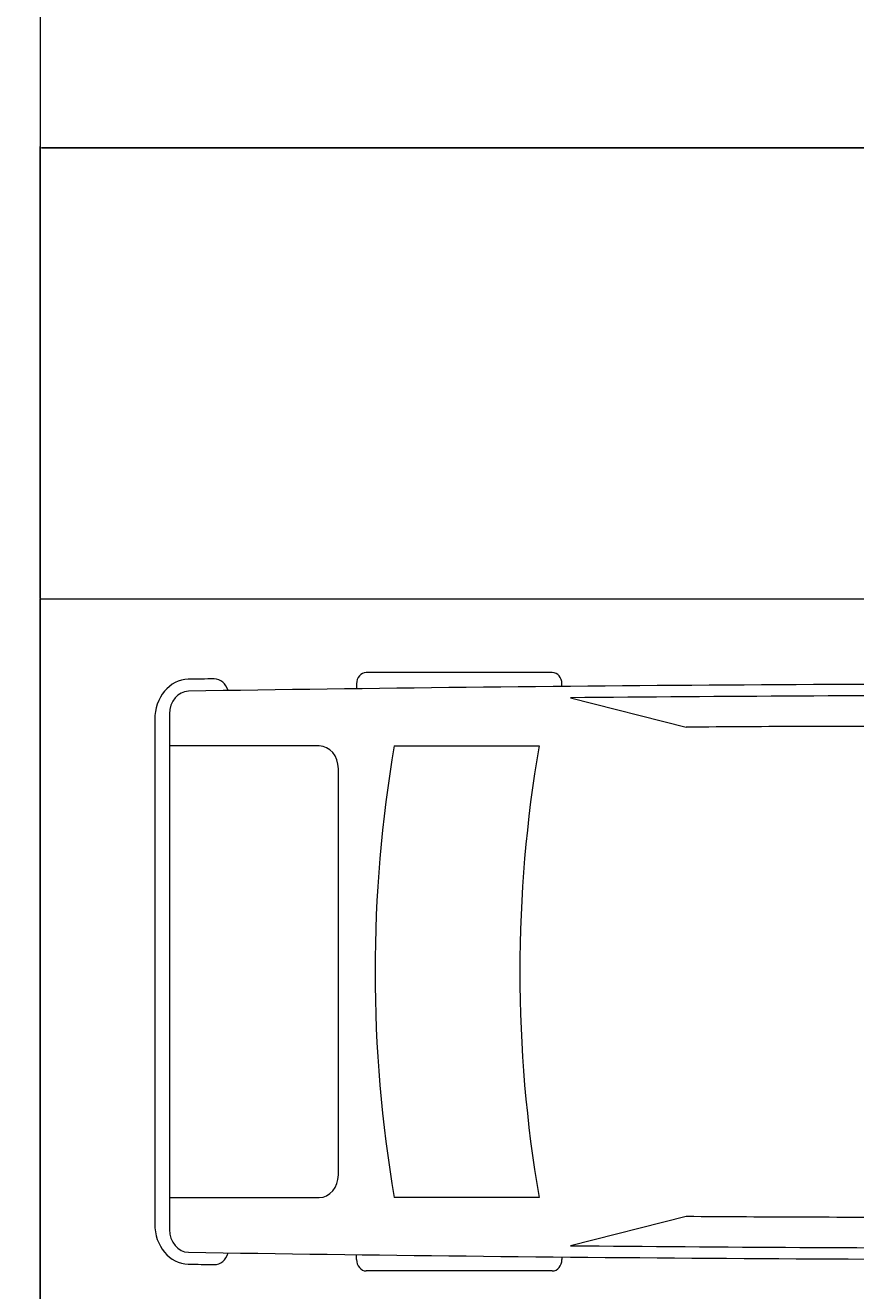
# Model space of a CAD drawing. Units: inches. Extents: x -46 to 1145, y -527 to 760.
# Tile 4 of 57: x 272 to 380, y -435 to -270. Entities that reach past the tile are written whole.
import ezdxf

# ---------------------------------------------------------------- set-up
doc = ezdxf.new("R2010")
doc.units = ezdxf.units.IN
doc.header["$MEASUREMENT"] = 0
for name, color, linetype, lineweight in [('A-ANNO-DIMS', 2, 'Continuous', 18), ('C-PKNG', 8, 'Continuous', 18), ('C-PKNG-VEHI', 8, 'Continuous', 13)]:
    doc.layers.add(name, color=color, linetype=linetype, lineweight=lineweight)
doc.styles.get("Standard").update_dxf_attribs({"font": 'arial.ttf'})
doc.dimstyles.get("Standard").update_dxf_attribs({"dimtxt": 0.18, "dimasz": 0.18, "dimexe": 0.18, "dimexo": 0.0625, "dimgap": 0.09, "dimtad": 0, "dimtih": 1, "dimtoh": 1, "dimdec": 0, "dimzin": 0, "dimdsep": 46, "dimlunit": 3, "dimtxsty": 'Standard', "dimcen": 0.09, "dimadec": 0, "dimazin": 0, "dimtfac": 1, "dimtdec": 0, "dimtofl": 0, "dimtmove": 0, "dimatfit": 3, "dimfxl": 1, "dimtolj": 1, "dimtzin": 0, "dimarcsym": 0})

# ---------------------------------------------------------------- blocks, each defined once
blk = doc.blocks.new('*U640')
for p, q in [((3472.1, 987.8), (4086.9, 987.8)), ((3440.5, 941.7), (3440.5, 950.2)), ((4118.5, 950.2), (4118.5, 934.1)), ((3411.6, 904.3), (3029.9, 807.2)), ((4736.4, -850.9), (4736.4, 850.9)), ((4785.3, -832.1), (4785.3, 832.1)), ((3515.9, 745.5), (3994.1, 745.5)), ((4736.4, 745.5), (4242, 745.5)), ((4178.7, 670.3), (4178.7, -670.3)), ((4736.4, -267.4), (4736.4, 267.4)), ((3994.1, -745.5), (3515.9, -745.5)), ((4242, -745.5), (4736.4, -745.5)), ((3411.6, -904.3), (3029.9, -807.2)), ((3440.5, -941.7), (3440.5, -950.2)), ((4118.5, -950.2), (4118.5, -934.1)), ((3472.1, -987.8), (4086.9, -987.8))]:
    blk.add_line(p, q)
for centre, major_axis, start_param, end_param in [((3472.1, 950.2), (0, -37.6), 3.141593, 4.712389), ((4086.9, 950.2), (0, 37.6), -1.570796, 0), ((4588, 910.3), (0, 56.4), -0.013017, 1.249894), ((1637.8, -268131.5), (0, 269121), -0.013397, -0.013017), ((4673.1, 832.1), (0, -133.3), 1.570796, 3.128196), ((1637.8, -268112.7), (0, 269062.9), -0.013397, 0.002797), ((4673.1, 850.9), (0, -75.2), 1.570796, 3.128196), ((1637.8, -268112.7), (0, -269025.3), 3.133765, 3.140441), ((2433, -93125.4), (0, -93935.2), 3.134049, 3.144098), ((433.9, 0), (0, 3734.3), 4.511394, 4.913384), ((912, 0), (0, 3734.3), 4.511394, 4.913384), ((4242, 670.3), (0, 75.2), 0, 1.570796), ((4242, -670.3), (0, -75.2), 4.712389, 6.283185), ((2433, 93125.4), (0, -93935.2), -0.002505, 0.007544), ((4673.1, -832.1), (0, -133.3), 0.013397, 1.570796), ((4673.1, -850.9), (0, 75.2), 3.15499, 4.712389), ((1637.8, 268112.7), (0, -269025.3), 0.001152, 0.007828), ((1637.8, 268112.7), (0, 269062.9), 3.138796, 3.15499), ((3472.1, -950.2), (0, -37.6), -1.570796, 0), ((4086.9, -950.2), (0, 37.6), 3.141593, 4.712389), ((4588, -910.3), (0, -56.4), -1.249894, 0.013017), ((1637.8, 268131.5), (0, 269121), 3.15461, 3.15499)]:
    blk.add_ellipse(centre, major_axis=major_axis, ratio=0.842304, start_param=start_param, end_param=end_param)
blk = doc.blocks.new('*D691')
at = {"layer": 'A-ANNO-DIMS', "color": 0, "lineweight": -2, "transparency": 16777216}
for p, q in [((273.52, -344.94), (273.52, -286.22)), ((273.7, -286.4), (387.23, -286.4)), ((501.55, -286.4), (388.02, -286.4)), ((501.73, -344.94), (501.73, -286.22))]:
    blk.add_line(p, q, dxfattribs=at)
at = {"layer": 'A-ANNO-DIMS', "color": 0, "transparency": 16777216}
for points in [[(273.7, -286.37), (273.7, -286.43), (273.52, -286.4)], [(501.55, -286.37), (501.55, -286.43), (501.73, -286.4)]]:
    blk.add_solid(points, dxfattribs=at)
at = {"layer": 'Defpoints', "color": 0, "transparency": 16777216}
for p in [(501.73, -286.4), (273.52, -345), (501.73, -345)]:
    blk.add_point(p, dxfattribs=at)
at = {"layer": 'A-ANNO-DIMS', "color": 0, "transparency": 16777216, "insert": (387.62, -286.4), "char_height": 0.18, "attachment_point": 5}
blk.add_mtext('\\A1;228.2', dxfattribs=at)
blk = doc.blocks.new('*D702')
at = {"layer": 'A-ANNO-DIMS', "color": 0, "lineweight": -2, "transparency": 16777216}
for p, q in [((189.63, -39.48), (1145.34, -39.48)), ((1145.16, -39.66), (1145.16, -249.3)), ((1145.16, -459.3), (1145.16, -249.66)), ((183.63, -459.48), (1145.34, -459.48))]:
    blk.add_line(p, q, dxfattribs=at)
at = {"layer": 'A-ANNO-DIMS', "color": 0, "transparency": 16777216}
for points in [[(1145.13, -39.66), (1145.19, -39.66), (1145.16, -39.48)], [(1145.13, -459.3), (1145.19, -459.3), (1145.16, -459.48)]]:
    blk.add_solid(points, dxfattribs=at)
at = {"layer": 'Defpoints', "color": 0, "transparency": 16777216}
for p in [(189.56, -39.48), (1145.16, -39.48), (183.56, -459.48)]:
    blk.add_point(p, dxfattribs=at)
at = {"layer": 'A-ANNO-DIMS', "color": 0, "transparency": 16777216, "insert": (1145.16, -249.48), "char_height": 0.18, "attachment_point": 5}
blk.add_mtext('\\A1;420', dxfattribs=at)

msp = doc.modelspace()

# ---------------------------------------------------------------- linework, layer by layer
at = {"layer": 'C-PKNG'}
msp.add_line((273.5156, -39.4824), (273.5156, -459.4824), dxfattribs=at)
msp.add_lwpolyline([(501.7297, -443.2988), (273.5156, -443.2988), (273.5156, -345.0009), (501.7297, -345.0009)], close=True, dxfattribs=at)

# ---------------------------------------------------------------- block references
at = {"layer": 'C-PKNG-VEHI', "xscale": 0.0393700787401575, "yscale": 0.0393700787401575, "zscale": 0.0393700787401575, "rotation": 180}
msp.add_blockref('*U640', (476.808, -393.4831), dxfattribs=at)

# ---------------------------------------------------------------- dimensions: what is measured, and where the dimension line sits
at = {"layer": 'A-ANNO-DIMS'}
dim = msp.add_linear_dim(base=(1145.1637, -39.4824), p1=(183.5637, -459.4824), p2=(189.5637, -39.4824), angle=90, dimstyle='Standard', override={"dimdec": 0, "dimlfac": 1, "dimrnd": 0, "dimzin": 0, "dimdsep": 46, "dimlunit": 2}, dxfattribs=at)
dim.commit()
dim.dimension.update_dxf_attribs({"geometry": '*D702', "text_midpoint": (1145.1637, -249.4824)})
dim = msp.add_linear_dim(base=(501.7297, -286.4009), p1=(273.5156, -345.0009), p2=(501.7297, -345.0009), dimstyle='Standard', override={"dimdec": 1, "dimlfac": 1, "dimrnd": 0, "dimzin": 0, "dimdsep": 46, "dimlunit": 2}, dxfattribs=at)
dim.commit()
dim.dimension.update_dxf_attribs({"geometry": '*D691', "text_midpoint": (387.6227, -286.4009)})

doc.saveas('drawing.dxf')
